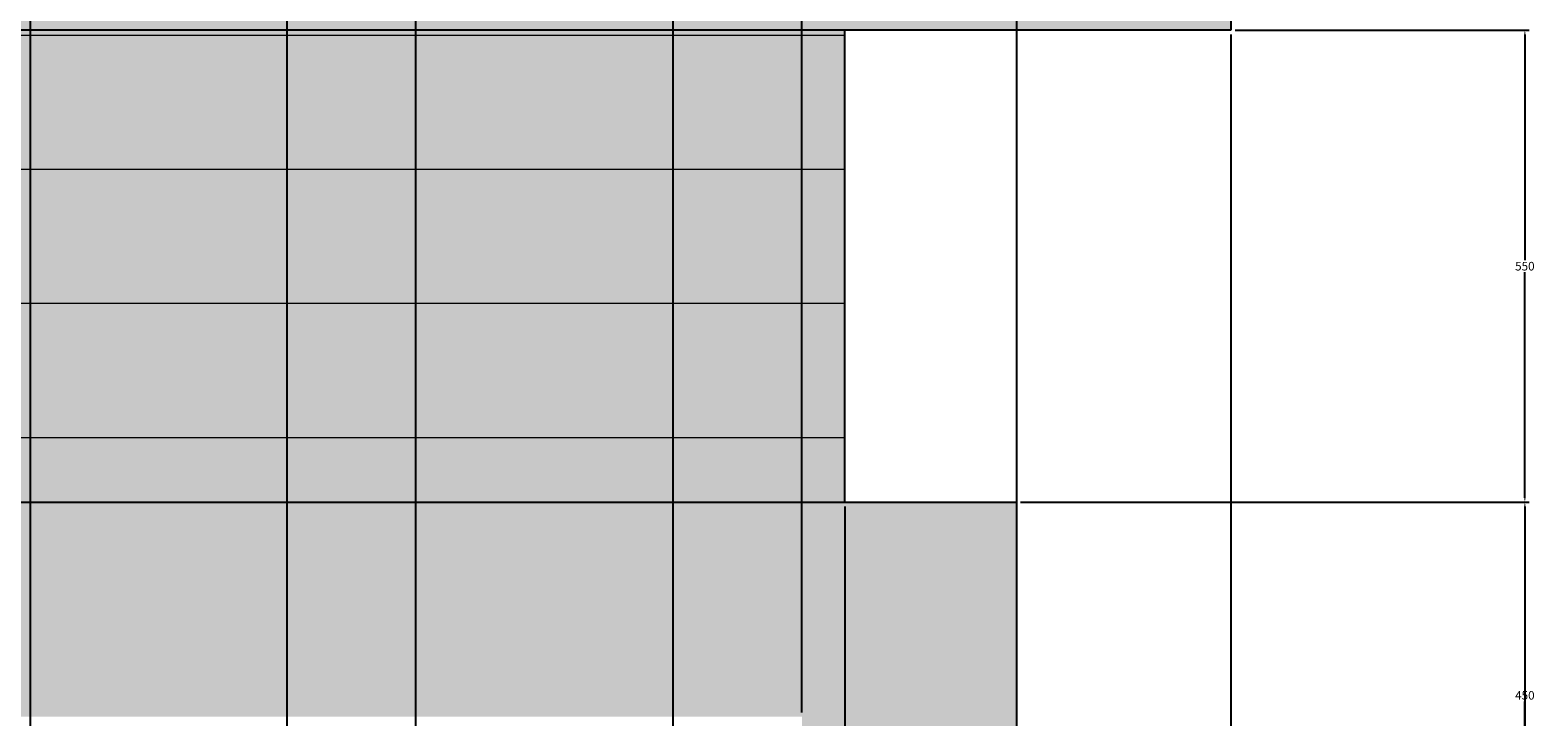
# Model space of a CAD drawing. Units: millimetres. Extents: x 2970 to 7764, y 2196 to 7505.
# Tile 10 of 13: x 6006 to 7764, y 4206 to 5006. Entities that reach past the tile are written whole.
import ezdxf

# ---------------------------------------------------------------- set-up
doc = ezdxf.new("R2010")
doc.units = ezdxf.units.MM
doc.header["$MEASUREMENT"] = 0
for name, color, linetype, lineweight in [('A-ANNO-DIMS', 2, 'Continuous', 18), ('A-ELEV', 7, 'Continuous', 25), ('A-ELEV-PATT', 8, 'Continuous', 13)]:
    doc.layers.add(name, color=color, linetype=linetype, lineweight=lineweight)
doc.styles.get("Standard").update_dxf_attribs({"font": 'arial.ttf'})
doc.dimstyles.get("Standard").update_dxf_attribs({"dimtxt": 10, "dimasz": 5, "dimexe": 5, "dimexo": 5, "dimgap": 2, "dimtad": 0, "dimtih": 1, "dimtoh": 1, "dimdec": 0, "dimzin": 0, "dimdsep": 46, "dimtxsty": 'Standard', "dimcen": 2, "dimadec": 0, "dimazin": 0, "dimtfac": 1, "dimtdec": 0, "dimtofl": 0, "dimtmove": 0, "dimatfit": 3, "dimfxl": 1, "dimtolj": 1, "dimtzin": 0, "dimarcsym": 0})

# ---------------------------------------------------------------- blocks, each defined once
blk = doc.blocks.new('*D30')
at = {"layer": 'A-ANNO-DIMS', "color": 0, "lineweight": -2, "transparency": 16777216}
for p, q in [((7160.5, 4455.8), (7753.5, 4455.8)), ((7748.5, 4450.8), (7748.5, 3707.9)), ((7748.5, 2950.8), (7748.5, 3693.7)), ((7510.5, 2945.8), (7753.5, 2945.8))]:
    blk.add_line(p, q, dxfattribs=at)
at = {"layer": 'A-ANNO-DIMS', "color": 0, "transparency": 16777216}
for points in [[(7747.7, 4450.8), (7749.3, 4450.8), (7748.5, 4455.8)], [(7747.7, 2950.8), (7749.3, 2950.8), (7748.5, 2945.8)]]:
    blk.add_solid(points, dxfattribs=at)
at = {"layer": 'Defpoints', "color": 0, "transparency": 16777216}
for p in [(7155.5, 4455.8), (7748.5, 4455.8), (7505.5, 2945.8)]:
    blk.add_point(p, dxfattribs=at)
at = {"layer": 'A-ANNO-DIMS', "color": 0, "transparency": 16777216, "insert": (7748.5, 3700.8), "char_height": 10, "attachment_point": 5}
blk.add_mtext('\\A1;1510', dxfattribs=at)
blk = doc.blocks.new('*D31')
at = {"layer": 'A-ANNO-DIMS', "color": 0, "lineweight": -2, "transparency": 16777216}
for p, q in [((7410.5, 5005.8), (7753.5, 5005.8)), ((7748.5, 5000.8), (7748.5, 4737.9)), ((7748.5, 4460.8), (7748.5, 4723.7)), ((7160.5, 4455.8), (7753.5, 4455.8))]:
    blk.add_line(p, q, dxfattribs=at)
at = {"layer": 'A-ANNO-DIMS', "color": 0, "transparency": 16777216}
for points in [[(7747.7, 5000.8), (7749.3, 5000.8), (7748.5, 5005.8)], [(7747.7, 4460.8), (7749.3, 4460.8), (7748.5, 4455.8)]]:
    blk.add_solid(points, dxfattribs=at)
at = {"layer": 'Defpoints', "color": 0, "transparency": 16777216}
for p in [(7405.5, 5005.8), (7748.5, 5005.8), (7155.5, 4455.8)]:
    blk.add_point(p, dxfattribs=at)
at = {"layer": 'A-ANNO-DIMS', "color": 0, "transparency": 16777216, "insert": (7748.5, 4730.8), "char_height": 10, "attachment_point": 5}
blk.add_mtext('\\A1;550', dxfattribs=at)
blk = doc.blocks.new('*D38')
at = {"layer": 'A-ANNO-DIMS', "color": 0, "lineweight": -2, "transparency": 16777216}
for p, q in [((6755.3, 4010.8), (6755.3, 7503.8)), ((6760.3, 7498.8), (6808.1, 7498.8)), ((6900.5, 7498.8), (6852.7, 7498.8)), ((6905.5, 4210.8), (6905.5, 7503.8))]:
    blk.add_line(p, q, dxfattribs=at)
at = {"layer": 'A-ANNO-DIMS', "color": 0, "transparency": 16777216}
for points in [[(6760.3, 7499.6), (6760.3, 7498), (6755.3, 7498.8)], [(6900.5, 7499.6), (6900.5, 7498), (6905.5, 7498.8)]]:
    blk.add_solid(points, dxfattribs=at)
at = {"layer": 'Defpoints', "color": 0, "transparency": 16777216}
for p in [(6905.5, 7498.8), (6905.5, 4205.8), (6755.3, 4005.8)]:
    blk.add_point(p, dxfattribs=at)
at = {"layer": 'A-ANNO-DIMS', "color": 0, "transparency": 16777216, "insert": (6830.4, 7498.8), "char_height": 10, "attachment_point": 5}
blk.add_mtext('\\A1;150.23', dxfattribs=at)
blk = doc.blocks.new('*D39')
at = {"layer": 'A-ANNO-DIMS', "color": 0, "lineweight": -2, "transparency": 16777216}
for p, q in [((5955.3, 4010.8), (5955.3, 7503.8)), ((5960.3, 7498.8), (6117.2, 7498.8)), ((6300.3, 7498.8), (6143.3, 7498.8)), ((6305.3, 4010.8), (6305.3, 7503.8))]:
    blk.add_line(p, q, dxfattribs=at)
at = {"layer": 'A-ANNO-DIMS', "color": 0, "transparency": 16777216}
for points in [[(5960.3, 7499.6), (5960.3, 7498), (5955.3, 7498.8)], [(6300.3, 7499.6), (6300.3, 7498), (6305.3, 7498.8)]]:
    blk.add_solid(points, dxfattribs=at)
at = {"layer": 'Defpoints', "color": 0, "transparency": 16777216}
for p in [(6305.3, 7498.8), (5955.3, 4005.8), (6305.3, 4005.8)]:
    blk.add_point(p, dxfattribs=at)
at = {"layer": 'A-ANNO-DIMS', "color": 0, "transparency": 16777216, "insert": (6130.3, 7498.8), "char_height": 10, "attachment_point": 5}
blk.add_mtext('\\A1;350', dxfattribs=at)
blk = doc.blocks.new('*D40')
at = {"layer": 'A-ANNO-DIMS', "color": 0, "lineweight": -2, "transparency": 16777216}
for p, q in [((6305.3, 4010.8), (6305.3, 7503.8)), ((6310.3, 7498.8), (6367.7, 7498.8)), ((6450.3, 7498.8), (6392.8, 7498.8)), ((6455.3, 4010.8), (6455.3, 7503.8))]:
    blk.add_line(p, q, dxfattribs=at)
at = {"layer": 'A-ANNO-DIMS', "color": 0, "transparency": 16777216}
for points in [[(6310.3, 7499.6), (6310.3, 7498), (6305.3, 7498.8)], [(6450.3, 7499.6), (6450.3, 7498), (6455.3, 7498.8)]]:
    blk.add_solid(points, dxfattribs=at)
at = {"layer": 'Defpoints', "color": 0, "transparency": 16777216}
for p in [(6455.3, 7498.8), (6305.3, 4005.8), (6455.3, 4005.8)]:
    blk.add_point(p, dxfattribs=at)
at = {"layer": 'A-ANNO-DIMS', "color": 0, "transparency": 16777216, "insert": (6380.3, 7498.8), "char_height": 10, "attachment_point": 5}
blk.add_mtext('\\A1;150', dxfattribs=at)
blk = doc.blocks.new('*D41')
at = {"layer": 'A-ANNO-DIMS', "color": 0, "lineweight": -2, "transparency": 16777216}
for p, q in [((6455.3, 4010.8), (6455.3, 7503.8)), ((6460.3, 7498.8), (6592.2, 7498.8)), ((6750.3, 7498.8), (6618.3, 7498.8)), ((6755.3, 4010.8), (6755.3, 7503.8))]:
    blk.add_line(p, q, dxfattribs=at)
at = {"layer": 'A-ANNO-DIMS', "color": 0, "transparency": 16777216}
for points in [[(6460.3, 7499.6), (6460.3, 7498), (6455.3, 7498.8)], [(6750.3, 7499.6), (6750.3, 7498), (6755.3, 7498.8)]]:
    blk.add_solid(points, dxfattribs=at)
at = {"layer": 'Defpoints', "color": 0, "transparency": 16777216}
for p in [(6755.3, 7498.8), (6455.3, 4005.8), (6755.3, 4005.8)]:
    blk.add_point(p, dxfattribs=at)
at = {"layer": 'A-ANNO-DIMS', "color": 0, "transparency": 16777216, "insert": (6605.3, 7498.8), "char_height": 10, "attachment_point": 5}
blk.add_mtext('\\A1;300', dxfattribs=at)
blk = doc.blocks.new('*D42')
at = {"layer": 'A-ANNO-DIMS', "color": 0, "lineweight": -2, "transparency": 16777216}
for p, q in [((6955.5, 4450.8), (6955.5, 2197.8)), ((7155.5, 4450.8), (7155.5, 2197.8)), ((6960.5, 2202.8), (7042.4, 2202.8)), ((7150.5, 2202.8), (7068.6, 2202.8))]:
    blk.add_line(p, q, dxfattribs=at)
at = {"layer": 'A-ANNO-DIMS', "color": 0, "transparency": 16777216}
for points in [[(6960.5, 2203.6), (6960.5, 2202), (6955.5, 2202.8)], [(7150.5, 2203.6), (7150.5, 2202), (7155.5, 2202.8)]]:
    blk.add_solid(points, dxfattribs=at)
at = {"layer": 'Defpoints', "color": 0, "transparency": 16777216}
for p in [(6955.5, 4455.8), (7155.5, 4455.8), (7155.5, 2202.8)]:
    blk.add_point(p, dxfattribs=at)
at = {"layer": 'A-ANNO-DIMS', "color": 0, "transparency": 16777216, "insert": (7055.5, 2202.8), "char_height": 10, "attachment_point": 5}
blk.add_mtext('\\A1;200', dxfattribs=at)
blk = doc.blocks.new('*D52')
at = {"layer": 'A-ANNO-DIMS', "color": 0, "lineweight": -2, "transparency": 16777216}
for p, q in [((7160.5, 4455.8), (7753.5, 4455.8)), ((7748.5, 4450.8), (7748.5, 4237.9)), ((7748.5, 4010.8), (7748.5, 4223.7)), ((6760.3, 4005.8), (7753.5, 4005.8))]:
    blk.add_line(p, q, dxfattribs=at)
at = {"layer": 'A-ANNO-DIMS', "color": 0, "transparency": 16777216}
for points in [[(7747.7, 4450.8), (7749.3, 4450.8), (7748.5, 4455.8)], [(7747.7, 4010.8), (7749.3, 4010.8), (7748.5, 4005.8)]]:
    blk.add_solid(points, dxfattribs=at)
at = {"layer": 'Defpoints', "color": 0, "transparency": 16777216}
for p in [(7155.5, 4455.8), (7748.5, 4455.8), (6755.3, 4005.8)]:
    blk.add_point(p, dxfattribs=at)
at = {"layer": 'A-ANNO-DIMS', "color": 0, "transparency": 16777216, "insert": (7748.5, 4230.8), "char_height": 10, "attachment_point": 5}
blk.add_mtext('\\A1;450', dxfattribs=at)
blk = doc.blocks.new('*D59')
at = {"layer": 'A-ANNO-DIMS', "color": 0, "lineweight": -2, "transparency": 16777216}
for p, q in [((6005.5, 5250.8), (6005.5, 2197.8)), ((7155.5, 5250.8), (7155.5, 2197.8)), ((6010.5, 2202.8), (6564.1, 2202.8)), ((7150.5, 2202.8), (6596.9, 2202.8))]:
    blk.add_line(p, q, dxfattribs=at)
at = {"layer": 'A-ANNO-DIMS', "color": 0, "transparency": 16777216}
for points in [[(6010.5, 2203.6), (6010.5, 2202), (6005.5, 2202.8)], [(7150.5, 2203.6), (7150.5, 2202), (7155.5, 2202.8)]]:
    blk.add_solid(points, dxfattribs=at)
at = {"layer": 'Defpoints', "color": 0, "transparency": 16777216}
for p in [(6005.5, 5255.8), (7155.5, 5255.8), (7155.5, 2202.8)]:
    blk.add_point(p, dxfattribs=at)
at = {"layer": 'A-ANNO-DIMS', "color": 0, "transparency": 16777216, "insert": (6580.5, 2202.8), "char_height": 10, "attachment_point": 5}
blk.add_mtext('\\A1;1150', dxfattribs=at)
blk = doc.blocks.new('*D60')
at = {"layer": 'A-ANNO-DIMS', "color": 0, "lineweight": -2, "transparency": 16777216}
for p, q in [((7155.5, 5250.8), (7155.5, 2197.8)), ((7405.5, 5000.8), (7405.5, 2197.8)), ((7160.5, 2202.8), (7267.4, 2202.8)), ((7400.5, 2202.8), (7293.6, 2202.8))]:
    blk.add_line(p, q, dxfattribs=at)
at = {"layer": 'A-ANNO-DIMS', "color": 0, "transparency": 16777216}
for points in [[(7160.5, 2203.6), (7160.5, 2202), (7155.5, 2202.8)], [(7400.5, 2203.6), (7400.5, 2202), (7405.5, 2202.8)]]:
    blk.add_solid(points, dxfattribs=at)
at = {"layer": 'Defpoints', "color": 0, "transparency": 16777216}
for p in [(7155.5, 5255.8), (7405.5, 5005.8), (7405.5, 2202.8)]:
    blk.add_point(p, dxfattribs=at)
at = {"layer": 'A-ANNO-DIMS', "color": 0, "transparency": 16777216, "insert": (7280.5, 2202.8), "char_height": 10, "attachment_point": 5}
blk.add_mtext('\\A1;250', dxfattribs=at)

msp = doc.modelspace()

# ---------------------------------------------------------------- hatches: boundary and pattern name
at = {"layer": 'A-ELEV-PATT'}
h = msp.add_hatch(color=256, dxfattribs=at)
h.dxf.hatch_style = 1
h.paths.add_polyline_path([(6405.5, 7255.789), (4305.5, 7255.789), (4305.5, 6505.789), (3730.5, 6505.789), (3730.5, 4205.789), (3730.5, 2945.789), (3730.5, 2895.789), (3830.5, 2895.789), (3830.5, 4205.789), (3830.5, 6405.789), (4405.5, 6405.789), (4405.5, 4205.789), (6905.5, 4205.789), (6905.5, 2945.789), (6905.5, 2845.789), (7155.5, 2845.789), (7155.5, 2945.789), (7155.5, 4205.789), (7155.5, 4455.789), (4555.5, 4455.789), (4555.5, 6505.789), (4555.5, 7005.789), (6155.5, 7005.789), (6155.5, 6755.789), (6405.5, 6755.789)])
h.paths.add_polyline_path([(7405.5, 6755.789), (6155.5, 6755.789), (5755.5, 6755.789), (5755.5, 5005.789), (7405.5, 5005.789)])
h.paths.add_polyline_path([(7155.5, 6505.789), (7155.5, 5255.789), (6005.5, 5255.789), (6005.5, 6505.789)], flags=16)
h.paths.add_polyline_path([(6105.5, 5520.789), (6105.5, 6055.789), (6455.5, 6055.789), (6455.5, 5520.789), (6655.5, 5520.789), (6655.5, 5605.789), (6655.5, 5955.789), (6955.5, 5955.789), (6955.5, 5605.789), (6955.5, 5520.789)], flags=0)
h.paths.add_polyline_path([(6425.5, 5755.789), (6425.5, 5655.789), (6425.5, 5555.789), (6405.5, 5555.789), (6405.5, 5755.789)], flags=0)
h.paths.add_polyline_path([(6955.5, 5505.789), (6955.5, 5405.789), (6655.5, 5405.789), (6655.5, 5505.789)], flags=0)
h = msp.add_hatch(color=256, dxfattribs=at)
h.set_gradient(color1=(147, 149, 152), color2=(199, 200, 202), name='CURVED')
h.paths.add_polyline_path([(6955.5, 4455.789), (6955.5, 5005.789), (5755.5, 5005.789), (5755.5, 6755.789), (6155.5, 6755.789), (6155.5, 7005.789), (4555.5, 7005.789), (4555.5, 6505.789), (4555.5, 4455.789)])
h.paths.add_polyline_path([(5015.81, 5462.49), (5015.81, 6062.49), (5455.81, 6062.49), (5455.81, 5462.49)], flags=16)
h.paths.add_polyline_path([(5035.81, 5482.49), (5035.81, 6042.49), (5155.81, 6042.49), (5155.81, 5482.49)], flags=0)
h.paths.add_polyline_path([(5175.81, 5482.49), (5175.81, 6042.49), (5295.81, 6042.49), (5295.81, 5482.49)], flags=0)
h.paths.add_polyline_path([(5315.81, 5482.49), (5315.81, 6042.49), (5435.81, 6042.49), (5435.81, 5482.49)], flags=0)
h.paths.add_polyline_path([(4865.81, 6162.49), (4865.81, 6212.49), (4840.81, 6212.49), (4840.81, 6237.49), (5630.81, 6237.49), (5630.81, 6212.49), (5605.81, 6212.49), (5605.81, 6162.49), (5015.81, 6162.49)], flags=16)
h = msp.add_hatch(dxfattribs=at)
h.set_pattern_fill('ANSI31', color=256, scale=1250, angle=135, style=0)
h.paths.add_polyline_path([(5755.5, 6755.789), (6155.5, 6755.789), (6155.5, 7005.789), (4555.5, 7005.789), (4555.5, 6505.789), (4555.5, 4455.789), (6955.5, 4455.789), (6955.5, 5005.789), (5755.5, 5005.789)])
h.paths.add_polyline_path([(5015.81, 5462.49), (5015.81, 6062.49), (5455.81, 6062.49), (5455.81, 5462.49)], flags=16)
h.paths.add_polyline_path([(5035.81, 5482.49), (5035.81, 6042.49), (5155.81, 6042.49), (5155.81, 5482.49)], flags=0)
h.paths.add_polyline_path([(5175.81, 5482.49), (5175.81, 6042.49), (5295.81, 6042.49), (5295.81, 5482.49)], flags=0)
h.paths.add_polyline_path([(5315.81, 5482.49), (5315.81, 6042.49), (5435.81, 6042.49), (5435.81, 5482.49)], flags=0)
h.paths.add_polyline_path([(4865.81, 6162.49), (4865.81, 6212.49), (4840.81, 6212.49), (4840.81, 6237.49), (5630.81, 6237.49), (5630.81, 6212.49), (5605.81, 6212.49), (5605.81, 6162.49), (5015.81, 6162.49)], flags=16)

# ---------------------------------------------------------------- linework, layer by layer
at = {"layer": 'A-ELEV'}
for p, q in [((7405.5, 6755.789), (7405.5, 5005.789)), ((7405.5, 5005.789), (5755.5, 5005.789)), ((6955.5, 4455.789), (6955.5, 5005.789)), ((4555.5, 4455.789), (7155.5, 4455.789)), ((7155.5, 4455.789), (7155.5, 4205.789))]:
    msp.add_line(p, q, dxfattribs=at)

# ---------------------------------------------------------------- dimensions: what is measured, and where the dimension line sits
at = {"layer": 'A-ANNO-DIMS'}
for base, p1, p2, override, picture, middle in [((6305.271, 7498.789), (5955.271, 4005.789), (6305.271, 4005.789), {"dimdec": 0, "dimlfac": 1, "dimrnd": 0, "dimzin": 0, "dimdsep": 46, "dimlunit": 2}, '*D39', (6130.271, 7498.789)), ((6455.271, 7498.789), (6305.271, 4005.789), (6455.271, 4005.789), {"dimdec": 0, "dimlfac": 1, "dimrnd": 0, "dimzin": 0, "dimdsep": 46, "dimlunit": 2}, '*D40', (6380.271, 7498.789)), ((6755.271, 7498.789), (6455.271, 4005.789), (6755.271, 4005.789), {"dimdec": 0, "dimlfac": 1, "dimrnd": 0, "dimzin": 0, "dimdsep": 46, "dimlunit": 2}, '*D41', (6605.271, 7498.789)), ((6905.5, 7498.789), (6755.271, 4005.789), (6905.5, 4205.789), {"dimdec": 2, "dimlfac": 1, "dimrnd": 0, "dimzin": 0, "dimdsep": 46, "dimlunit": 2}, '*D38', (6830.386, 7498.789)), ((7155.5, 2202.789), (6005.5, 5255.789), (7155.5, 5255.789), {"dimdec": 0, "dimlfac": 1, "dimrnd": 0, "dimzin": 0, "dimdsep": 46, "dimlunit": 2}, '*D59', (6580.5, 2202.789)), ((7405.5, 2202.789), (7155.5, 5255.789), (7405.5, 5005.789), {"dimdec": 0, "dimlfac": 1, "dimrnd": 0, "dimzin": 0, "dimdsep": 46, "dimlunit": 2}, '*D60', (7280.5, 2202.789)), ((7155.5, 2202.789), (6955.5, 4455.789), (7155.5, 4455.789), {"dimdec": 0, "dimlfac": 1, "dimrnd": 0, "dimzin": 0, "dimdsep": 46, "dimlunit": 2}, '*D42', (7055.5, 2202.789))]:
    dim = msp.add_linear_dim(base=base, p1=p1, p2=p2, dimstyle='Standard', override=override, dxfattribs=at)
    dim.commit()
    dim.dimension.update_dxf_attribs({"geometry": picture, "text_midpoint": middle})
for base, p1, p2, picture, middle in [((7748.5, 5005.789), (7155.5, 4455.789), (7405.5, 5005.789), '*D31', (7748.5, 4730.789)), ((7748.5, 4455.789), (6755.271, 4005.789), (7155.5, 4455.789), '*D52', (7748.5, 4230.789)), ((7748.5, 4455.789), (7505.5, 2945.789), (7155.5, 4455.789), '*D30', (7748.5, 3700.789))]:
    dim = msp.add_linear_dim(base=base, p1=p1, p2=p2, angle=90, dimstyle='Standard', override={"dimdec": 0, "dimlfac": 1, "dimrnd": 0, "dimzin": 0, "dimdsep": 46, "dimlunit": 2}, dxfattribs=at)
    dim.commit()
    dim.dimension.update_dxf_attribs({"geometry": picture, "text_midpoint": middle})

doc.saveas('drawing.dxf')
